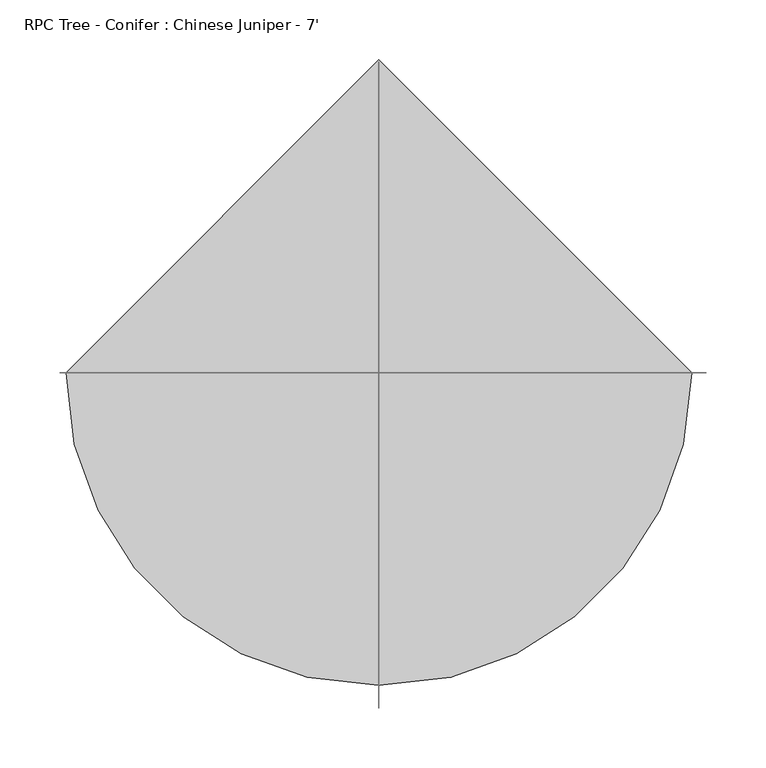
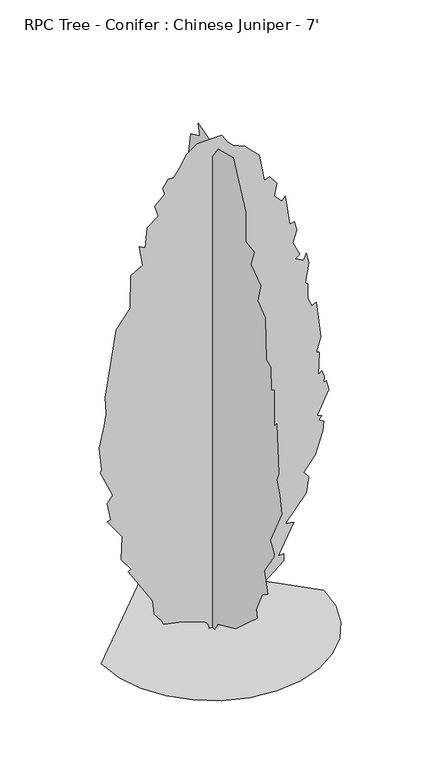
"""IFC4 building model written with IfcOpenShell, lengths in millimetres: geographic element geometry, RPC Tree - Conifer : Chinese Juniper - 7'."""

from ifc_helpers import new_model, si_unit, origin, place, context, project, spatial, triangles, source, transform, mapped, element, save


def rpc_tree_conifer_chinese_juniper_7_393522d0(model_context):
    return source(origin(), model_context, "Body", "Tessellation", [
        triangles([(-8.2115105, 4e-07, 7e-07), (-10.2054897, -2e-07, 10.2512547), (-15.5856334, -3e-07, 17.3665431), (-70.5263002, 9e-07, 37.5861687), (-115.1591772, 2.2e-06, 47.0570614), (-119.4371319, 1.8e-06, 57.7518028), (-136.6736253, 1.2e-06, 79.8164853), (-140.8269055, -6e-07, 113.3646283), (-147.2442646, -1.1e-06, 126.1983471), (-198.5785585, -3.7e-06, 207.4780153), (-191.9368127, -4.2e-06, 211.4694686), (-214.6502882, -5.1e-06, 243.3110025), (-212.3483212, -8.6e-06, 299.7877333), (-247.7749015, -9.9e-06, 348.6502304), (-239.2187014, -1.04e-05, 350.7881813), (-247.442509, -1.27e-05, 394.0118511), (-234.9398746, -1.42e-05, 410.6786754), (-264.8858484, -1.68e-05, 476.9874187), (-260.608475, -1.73e-05, 481.2647738), (-267.0252527, -2.04e-05, 539.0158636), (-255.4166953, -2.4e-05, 589.4023593), (-249.9128524, -2.59e-05, 618.1581259), (-252.0522749, -2.82e-05, 658.7983051), (-226.3851279, -3.89e-05, 819.2193998), (-194.3011851, -4.29e-05, 861.9989107), (-192.5667343, -4.77e-05, 941.8437464), (-164.3552296, -4.99e-05, 958.2521925), (-172.9114297, -5.25e-05, 1007.4470821), (-158.3085601, -5.26e-05, 999.0693958), (-153.6610604, -5.57e-05, 1048.0871887), (-127.992896, -5.8e-05, 1067.3375399), (-136.5488055, -5.93e-05, 1095.1441275), (-113.0201998, -6.16e-05, 1116.5338829), (-117.2981546, -6.23e-05, 1131.5068789), (-104.4644357, -6.4e-05, 1150.75723), (-91.6307169, -6.46e-05, 1150.75723), (-76.9059253, -6.64e-05, 1169.8754671), (-62.1436905, -6.87e-05, 1197.6268982), (-35.6577935, -7.09e-05, 1215.562286), (21.2925253, -7.34e-05, 1216.4577982), (34.5676234, -7.28e-05, 1195.6746918), (47.4013445, -7.26e-05, 1182.8411728), (75.9343458, -7.31e-05, 1170.756518), (109.4309567, -7.25e-05, 1135.784234), (122.2646755, -6.91e-05, 1069.4769442), (135.0983944, -6.99e-05, 1073.7542994), (150.7509364, -6.92e-05, 1051.3616255), (145.7928452, -6.73e-05, 1022.4200054), (162.9052272, -6.69e-05, 1003.1696543), (171.459974, -6.78e-05, 1011.7258907), (182.1555965, -6.39e-05, 939.000388), (192.8497476, -6.45e-05, 941.1397923), (198.6656353, -6.35e-05, 919.9503153), (189.1064986, -6.14e-05, 890.8737471), (205.683321, -6e-05, 855.5821512), (194.4753569, -5.91e-05, 848.8619946), (214.2395212, -5.93e-05, 838.469751), (220.6562988, -6.05e-05, 853.4427469), (227.0730947, -5.93e-05, 827.7755636), (218.5183479, -5.61e-05, 780.7186975), (224.6941883, -5.6e-05, 775.6371763), (223.8363918, -5.39e-05, 740.8927855), (233.4898723, -5.3e-05, 718.6887629), (244.1854949, -5.38e-05, 722.966118), (254.8796459, -4.89e-05, 633.1311218), (244.1854949, -4.64e-05, 598.9077747), (250.8461167, -4.65e-05, 596.6450131), (248.4628683, -4.31e-05, 541.1552679), (257.0190684, -4.39e-05, 547.5720637), (263.435846, -4.33e-05, 532.5990678), (261.2964417, -4.23e-05, 517.6275252), (267.7132194, -4.27e-05, 519.7654761), (274.1300152, -4.16e-05, 496.2377698), (246.3234458, -3.7e-05, 440.6246309), (257.0190684, -3.72e-05, 436.3472757), (250.6022726, -3.64e-05, 427.7910756), (261.2964417, -3.65e-05, 421.3742798), (259.0467062, -3.51e-05, 398.3211811), (242.0460724, -3.11e-05, 344.3713855), (214.2395212, -2.78e-05, 310.1480384), (227.0730947, -2.75e-05, 295.1750788), (220.0583157, -2.5e-05, 257.8093726), (171.459974, -1.92e-05, 196.7838643), (190.7117785, -1.99e-05, 194.64446), (154.3490271, -1.41e-05, 124.0593698), (167.1826006, -1.47e-05, 124.0593698), (167.1826006, -1.37e-05, 106.9476962), (73.0684915, -5e-06, 29.9453901), (73.0684915, -5.6e-06, 40.6401293), (8.9001324, -4e-07, 0.0), (0.1966717, 7.8795262, 7.43e-05), (0.1966726, 19.7034962, 8.1693335), (0.196674, 44.2417172, 17.1118166), (0.1966752, 101.9935201, 38.5012973), (0.1966777, 131.9389124, 66.3077123), (0.1966772, 119.1051936, 68.4466896), (0.1966821, 164.8828136, 134.4323286), (0.1966829, 151.1899903, 166.8378905), (0.1966848, 189.6907107, 222.4510112), (0.1966857, 185.4133374, 248.1181582), (0.1966884, 213.2184352, 282.3415053), (0.1966906, 222.5671197, 323.2748171), (0.1966899, 217.497262, 365.7611773), (0.1966937, 251.7206091, 417.0954712), (0.196696, 253.8585782, 468.4312185), (0.1966973, 241.5039725, 510.4414813), (0.1966988, 260.2753558, 577.5180193), (0.1966991, 243.164409, 601.045762), (0.1967011, 221.7746354, 669.4924198), (0.1967015, 236.7476313, 716.5493586), (0.1967038, 219.6352311, 784.9960527), (0.1967046, 198.2469109, 825.6361593), (0.1967056, 187.5512883, 911.1952538), (0.1967047, 174.717733, 904.7784943), (0.1967081, 174.717733, 981.7798988), (0.1967073, 149.0505769, 988.1966583), (0.1967064, 135.4715547, 1033.8878374), (0.1967077, 127.6609577, 1071.6163485), (0.1967077, 101.9935201, 1097.2835318), (0.1967105, 89.1598012, 1174.2863897), (0.1967074, 52.7974813, 1191.3973366), (0.1967088, 58.3198913, 1218.9310484), (0.1967058, 6.4850034, 1202.4064756), (0.1967064, 3.6015718, 1165.7302259), (0.1967046, -22.0658497, 1202.0929773), (0.1967026, -84.0954574, 1219.2039242), (0.1966981, -135.430478, 1114.3944786), (0.1966949, -135.430478, 1041.6704292), (0.1966931, -169.2603444, 1035.6484131), (0.1966921, -154.6806929, 996.7528948), (0.1966914, -195.9100986, 968.6081738), (0.1966899, -184.6266666, 924.0288454), (0.1966876, -214.571187, 900.499613), (0.1966852, -218.8499956, 797.8296444), (0.1966841, -236.3136462, 790.3794451), (0.1966815, -238.1003649, 733.6617588), (0.1966813, -250.9339384, 742.2164692), (0.1966797, -250.9339384, 652.381473), (0.1966775, -261.6280894, 665.2150646), (0.1966742, -270.1842895, 545.4340765), (0.1966737, -260.8965752, 525.0603201), (0.1966718, -274.4631163, 494.0983292), (0.1966719, -280.8799121, 451.3188183), (0.1966698, -235.9609424, 359.3443814), (0.1966681, -250.9339384, 333.6772345), (0.19667, -249.6682816, 324.6159416), (0.1966692, -210.2937954, 267.3699627), (0.1966664, -225.2667914, 218.1736379), (0.1966668, -201.7376135, 203.2006419), (0.1966679, -178.2098708, 151.8663571), (0.1966669, -182.4872442, 132.6152792), (0.196667, -139.7082874, 94.1141227), (0.1966672, -94.7901989, 53.4739935), (0.196669, -19.9265817, 19.2506486), (0.1966709, -9.2321167, 7.33e-05), (-261.6114116, 0.0, 8.53e-05), (-254.6895231, -59.9890391, 8.14e-05), (-234.9776085, -115.0794946, 7.72e-05), (-204.0533697, -163.6926428, 7.3e-05), (-163.4959797, -204.2500328, 6.88e-05), (-114.8828223, -235.1742717, 6.48e-05), (-59.7923669, -254.8861862, 6.12e-05), (0.1966828, -261.8080748, 5.82e-05), (60.1857113, -254.8861862, 5.6e-05), (115.2761668, -235.1742717, 5.48e-05), (163.889306, -204.2500328, 5.45e-05), (204.4466959, -163.6926428, 5.51e-05), (235.3709348, -115.0793492, 5.67e-05), (255.0828494, -59.9890391, 5.91e-05), (262.0047379, 2.29e-05, 6.24e-05), (0.1966369, 261.8080748, 8.94e-05)], [[57, 58, 59], [27, 28, 29], [87, 88, 89], [49, 50, 51], [13, 14, 15], [83, 84, 85], [74, 75, 76], [63, 64, 65], [68, 69, 70], [71, 72, 73], [9, 10, 11], [85, 86, 87], [85, 87, 89], [51, 52, 53], [54, 55, 56], [90, 1, 2], [66, 67, 68], [45, 46, 47], [17, 18, 19], [68, 70, 71], [45, 47, 48], [31, 32, 33], [76, 77, 78], [89, 90, 2], [89, 2, 3], [57, 59, 60], [51, 53, 54], [25, 26, 27], [39, 40, 41], [56, 57, 60], [71, 73, 74], [34, 35, 36], [33, 34, 36], [4, 5, 6], [60, 61, 62], [80, 81, 82], [38, 39, 41], [37, 38, 41], [37, 41, 42], [29, 30, 31], [15, 16, 17], [36, 37, 42], [33, 36, 42], [31, 33, 42], [31, 42, 43], [31, 43, 44], [31, 44, 45], [29, 31, 45], [29, 45, 48], [27, 29, 48], [25, 27, 48], [25, 48, 49], [25, 49, 51], [25, 51, 54], [25, 54, 56], [25, 56, 60], [25, 60, 62], [24, 25, 62], [23, 24, 62], [22, 23, 62], [22, 62, 63], [22, 63, 65], [22, 65, 66], [22, 66, 68], [21, 22, 68], [20, 21, 68], [19, 20, 68], [17, 19, 68], [17, 68, 71], [17, 71, 74], [15, 17, 74], [13, 15, 74], [13, 74, 76], [13, 76, 78], [13, 78, 79], [13, 79, 80], [12, 13, 80], [11, 12, 80], [9, 11, 80], [9, 80, 82], [9, 82, 83], [9, 83, 85], [9, 85, 89], [9, 89, 3], [9, 3, 4], [8, 9, 4], [8, 4, 6], [7, 8, 6], [138, 139, 140], [94, 95, 96], [136, 137, 138], [121, 122, 123], [112, 113, 114], [128, 129, 130], [121, 123, 124], [125, 126, 127], [124, 125, 127], [114, 115, 116], [147, 148, 149], [130, 131, 132], [124, 127, 128], [134, 135, 136], [154, 155, 91], [154, 91, 92], [150, 151, 152], [96, 97, 98], [119, 120, 121], [119, 121, 124], [119, 124, 128], [118, 119, 128], [117, 118, 128], [116, 117, 128], [116, 128, 130], [114, 116, 130], [114, 130, 132], [112, 114, 132], [112, 132, 133], [112, 133, 134], [112, 134, 136], [111, 112, 136], [110, 111, 136], [109, 110, 136], [109, 136, 138], [109, 138, 140], [109, 140, 141], [108, 109, 141], [107, 108, 141], [106, 107, 141], [105, 106, 141], [104, 105, 141], [103, 104, 141], [103, 141, 142], [103, 142, 143], [103, 143, 144], [102, 103, 144], [101, 102, 144], [100, 101, 144], [100, 144, 145], [100, 145, 146], [100, 146, 147], [100, 147, 149], [100, 149, 150], [100, 150, 152], [100, 152, 153], [100, 153, 154], [99, 100, 154], [98, 99, 154], [96, 98, 154], [96, 154, 92], [96, 92, 93], [96, 93, 94], [170, 171, 156], [169, 170, 156], [169, 156, 157], [168, 169, 157], [168, 157, 158], [168, 158, 159], [167, 168, 159], [166, 167, 159], [166, 159, 160], [166, 160, 161], [166, 161, 162], [166, 162, 163], [166, 163, 164], [166, 164, 165]], closed=False),
    ])


if __name__ == "__main__":
    model = new_model("IFC4")
    model_context = context("Model", 3, world=origin())
    ifc_project = project(units=[si_unit("LENGTHUNIT", "METRE", prefix="MILLI")], contexts=[model_context])
    site = spatial("IfcSite", under=ifc_project)
    building = spatial("IfcBuilding", under=site)
    placement = place(None, origin())
    rpc_tree_conifer_chinese_juniper_7_shape = rpc_tree_conifer_chinese_juniper_7_393522d0(model_context)
    element("IfcGeographicElement", 1, ObjectType="RPC Tree - Conifer : Chinese Juniper - 7'", at=placement, inside=building, context=model_context, shape_type="MappedRepresentation", body=[
        mapped(rpc_tree_conifer_chinese_juniper_7_shape, transform((0.0, 0.0, 0.0), x_axis=(1.0, 0.0, 0.0), y_axis=(0.0, 1.0, 0.0), z_axis=(0.0, 0.0, 1.0))),
    ])
    save(model, "model.ifc")

# Revit data of these elements
# Type "RPC Tree - Conifer : Chinese Juniper - 7'"
#   built-in parameter 1005198 = "{2, 15},{39, RPC-16-FUM3-UUQ0-UBF0-N000-ST1L-LVER-AU},{1, 0},{1, 0},{2, 13},{1, 8},{5, Color},{1, 0},{1, 0},{3, 0.8},{3, 0.8},{3, 0.8},{1, 8},{7, BBoxMin},{1, 0},{1, 0},{1, 0},{1, 0},{1, 0},{1, 8},{7, BBoxMax},{1, 0},{1, 0},{1, 0},{1, 0},{1, 0},{2, 11},{9, RPCTypeId},{1, 0},{1, 0},{39, RPC-16-FUM3-UUQ0-UBF0-N000-ST1L-LVER-AU},{1, 6},{14, RPCPlantHeight},{1, 0},{1, 0},{1, 7},{2, 11},{7, keyword},{1, 0},{1, 0},{34, :RPCs:Trees [General]:Geometry:RPC},{2, 11},{8, category},{1, 0},{1, 0},{15, Trees [General]},{2, 11},{12, LocalizedUID},{1, 0},{1, 0},{15, Chinese Juniper},{2, 14},{6, Height},{1, 0},{1, 0},{1, 7},{1, 2},{16, Cast Reflections},{1, 0},{1, 0},{1, 0},{1, 2},{12, Cast Shadows},{1, 0},{1, 0},{1, 1},{1, 2},{9, Lock View},{1, 0},{1, 0},{1, 0},{1, 4},{5, ViewC},{1, 0},{1, 0},{1, 0},{21, assetlibrary_base.fbx},{1, 5},"
#   built-in parameter 1005195 = "RPC-16-FUM3-UUQ0-UBF0-N000-ST1L-LVER-AU"
#   Type Comments = "Chinese Juniper"
#   Assembly Code = "G2050500"
#   Height = 4' - 0"
#   Description = (empty or 0)
#   Default Elevation = 0
